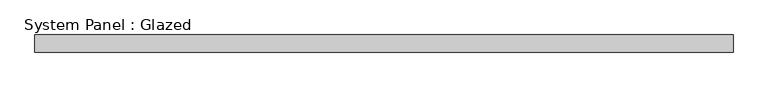
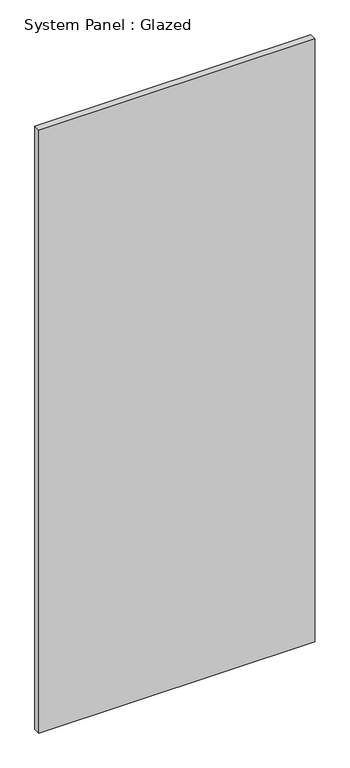
"""IFC4 building model written with IfcOpenShell, lengths in millimetres: plate geometry, System Panel : Glazed."""

from ifc_helpers import new_model, si_unit, origin, origin_with_axes, place, context, project, spatial, polyline, outline, extrude, source, transform, mapped, element, save


def system_panel_glazed_73690fa1(model_context):
    return source(origin(), model_context, "Body", "SweptSolid", [
        extrude(outline(polyline([(507.2023702, 19.05), (-507.2023702, 19.05), (-507.2023702, 44.45), (507.2023702, 44.45), (507.2023702, 19.05)])), origin_with_axes(), (0.0, 0.0, 1.0), 2343.15),
    ])


if __name__ == "__main__":
    model = new_model("IFC4")
    model_context = context("Model", 3, world=origin())
    ifc_project = project(units=[si_unit("LENGTHUNIT", "METRE", prefix="MILLI")], contexts=[model_context])
    site = spatial("IfcSite", under=ifc_project)
    building = spatial("IfcBuilding", under=site)
    placement = place(None, origin())
    system_panel_glazed_shape = system_panel_glazed_73690fa1(model_context)
    element("IfcPlate", 1, ObjectType="System Panel : Glazed", at=placement, inside=building, context=model_context, shape_type="MappedRepresentation", body=[
        mapped(system_panel_glazed_shape, transform((0.0, 0.0, 0.0), x_axis=(1.0, 0.0, 0.0), y_axis=(0.0, 1.0, 0.0), z_axis=(0.0, 0.0, 1.0))),
    ])
    save(model, "model.ifc")

# Revit data of these elements
# Type "System Panel : Glazed"
#   Construction Type Id = "GSP4R"
#   Analytic Construction = "1/8 in Pilkington single glazing"
#   Visual Light Transmittance = 0.9
#   Solar Heat Gain Coefficient = 0.86
#   Heat Transfer Coefficient (U) = 1.18115 BTU/(h·ft²·°F)
#   Define Thermal Properties by = 1
# Element 1 (IfcPlate, "System Panel : Glazed")
#   Materials on its faces: "Glass"
# Materials
#   "Glass": class "Glass", colour RGB 0 128 192, transparency 0.75, Description = "Soda Lime Glass", Cost = 0
